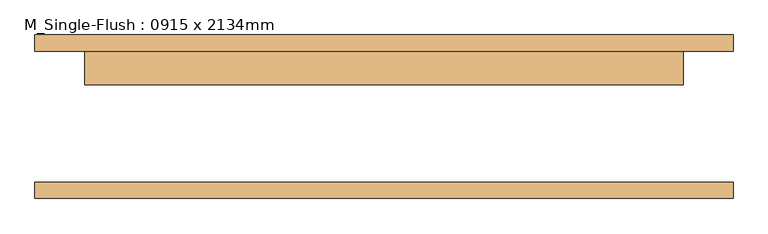
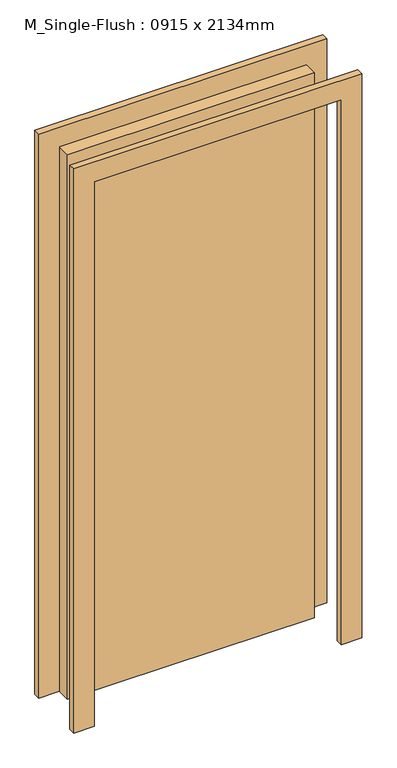
"""IFC4 building model written with IfcOpenShell, lengths in millimetres: door geometry, M_Single-Flush : 0915 x 2134mm."""

from ifc_helpers import new_model, si_unit, frame, origin, origin_with_axes, place, context, project, spatial, polyline, outline, extrude, source, transform, mapped, element, save


def m_single_flush_0915_x_2134mm_6a9e8738(model_context):
    return source(origin(), model_context, "Body", "SweptSolid", [
        extrude(outline(polyline([(2210.0, -533.5), (0.0, -533.5), (0.0, -457.5), (2134.0, -457.5), (2134.0, 457.5), (0.0, 457.5), (0.0, 533.5), (2210.0, 533.5), (2210.0, -533.5)])), frame((0.0, 100.0, 0.0), z_axis=(0.0, 1.0, 0.0), x_axis=(0.0, 0.0, 1.0)), (0.0, 0.0, 1.0), 25.0),
        extrude(outline(polyline([(2210.0, 533.5), (2210.0, -533.5), (0.0, -533.5), (0.0, -457.5), (2134.0, -457.5), (2134.0, 457.5), (0.0, 457.5), (0.0, 533.5), (2210.0, 533.5)])), frame((0.0, -125.0, 0.0), z_axis=(0.0, 1.0, 0.0), x_axis=(0.0, 0.0, 1.0)), (0.0, 0.0, 1.0), 25.0),
        extrude(outline(polyline([(457.5, 49.0), (-457.5, 49.0), (-457.5, 100.0), (457.5, 100.0), (457.5, 49.0)])), origin_with_axes(), (0.0, 0.0, 1.0), 2134.0),
    ])


if __name__ == "__main__":
    model = new_model("IFC4")
    model_context = context("Model", 3, world=origin())
    ifc_project = project(units=[si_unit("LENGTHUNIT", "METRE", prefix="MILLI")], contexts=[model_context])
    site = spatial("IfcSite", under=ifc_project)
    building = spatial("IfcBuilding", under=site)
    placement = place(None, origin())
    m_single_flush_0915_x_2134mm_shape = m_single_flush_0915_x_2134mm_6a9e8738(model_context)
    element("IfcDoor", 1, ObjectType="M_Single-Flush : 0915 x 2134mm", at=placement, inside=building, context=model_context, shape_type="MappedRepresentation", body=[
        mapped(m_single_flush_0915_x_2134mm_shape, transform((0.0, 0.0, 0.0), x_axis=(1.0, 0.0, 0.0), y_axis=(0.0, 1.0, 0.0), z_axis=(0.0, 0.0, 1.0))),
    ])
    save(model, "model.ifc")

# Revit data of these elements
# Type "M_Single-Flush : 0915 x 2134mm"
#   Type Mark = "15"
#   Thickness = 0' - 2.00787"
#   Height = 7' - 0.01575"
#   Trim Projection Ext = 0' - 0.98425"
#   Trim Projection Int = 0' - 0.98425"
#   Trim Width = 0' - 2.99213"
#   Width = 3' - 0.02362"
#   Door Material = Door - Panel
#   Frame Material = Door - Frame
#   Function = (empty or 0)
#   Wall Closure = (empty or 0)
# Element 1 (IfcDoor, "M_Single-Flush : 0915 x 2134mm")
#   Materials on its faces: "Door - Frame", "Door - Panel"
# Materials
#   "Door - Panel": class "Wood", colour RGB 114 82 51, transparency 0
#   "Door - Frame": colour RGB 153 76 43, transparency 0
